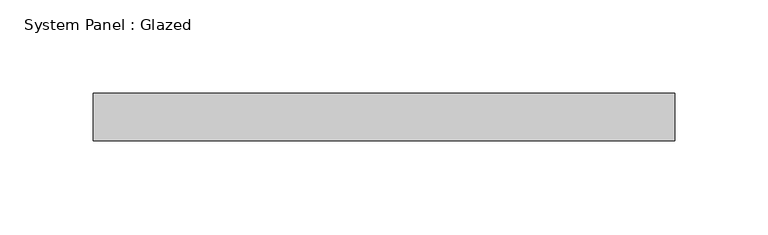
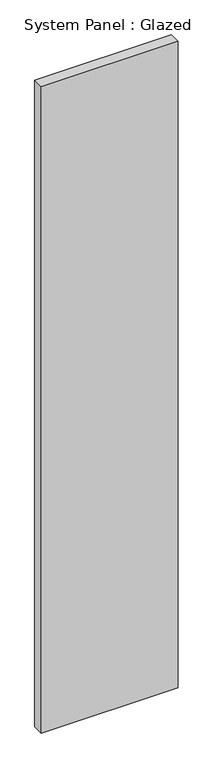
"""IFC4 building model written with IfcOpenShell, lengths in millimetres: plate geometry, System Panel : Glazed."""

from ifc_helpers import new_model, si_unit, origin, origin_with_axes, place, context, project, spatial, polyline, outline, extrude, source, transform, mapped, element, save


def system_panel_glazed_8f6bde40(model_context):
    return source(origin(), model_context, "Body", "SweptSolid", [
        extrude(outline(polyline([(155.575, 19.05), (-155.575, 19.05), (-155.575, 44.45), (155.575, 44.45), (155.575, 19.05)])), origin_with_axes(), (0.0, 0.0, 1.0), 1551.8095798),
    ])


if __name__ == "__main__":
    model = new_model("IFC4")
    model_context = context("Model", 3, world=origin())
    ifc_project = project(units=[si_unit("LENGTHUNIT", "METRE", prefix="MILLI")], contexts=[model_context])
    site = spatial("IfcSite", under=ifc_project)
    building = spatial("IfcBuilding", under=site)
    placement = place(None, origin())
    system_panel_glazed_shape = system_panel_glazed_8f6bde40(model_context)
    element("IfcPlate", 1, ObjectType="System Panel : Glazed", at=placement, inside=building, context=model_context, shape_type="MappedRepresentation", body=[
        mapped(system_panel_glazed_shape, transform((0.0, 0.0, 0.0), x_axis=(1.0, 0.0, 0.0), y_axis=(0.0, 1.0, 0.0), z_axis=(0.0, 0.0, 1.0))),
    ])
    save(model, "model.ifc")

# Revit data of these elements
# Type "System Panel : Glazed"
#   Construction Type Id = "GSP4R"
#   Analytic Construction = "1/8 in Pilkington single glazing"
#   Visual Light Transmittance = 0.9
#   Solar Heat Gain Coefficient = 0.86
#   Heat Transfer Coefficient (U) = 1.18115 BTU/(h·ft²·°F)
#   Define Thermal Properties by = 1
# Element 1 (IfcPlate, "System Panel : Glazed")
#   Materials on its faces: "Glass"
# Materials
#   "Glass": class "Glass", colour RGB 0 128 192, transparency 0.75, Description = "Soda Lime Glass", Cost = 0
